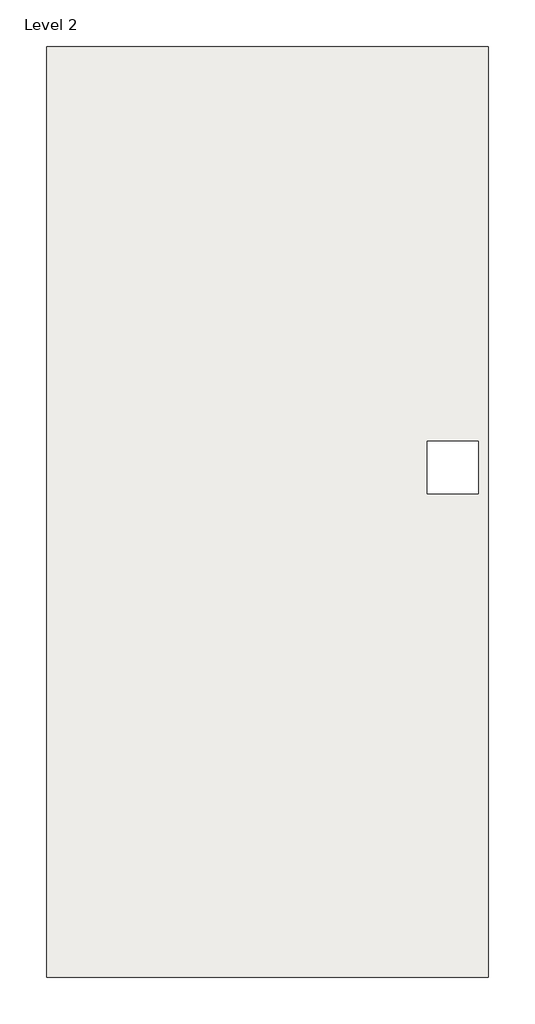
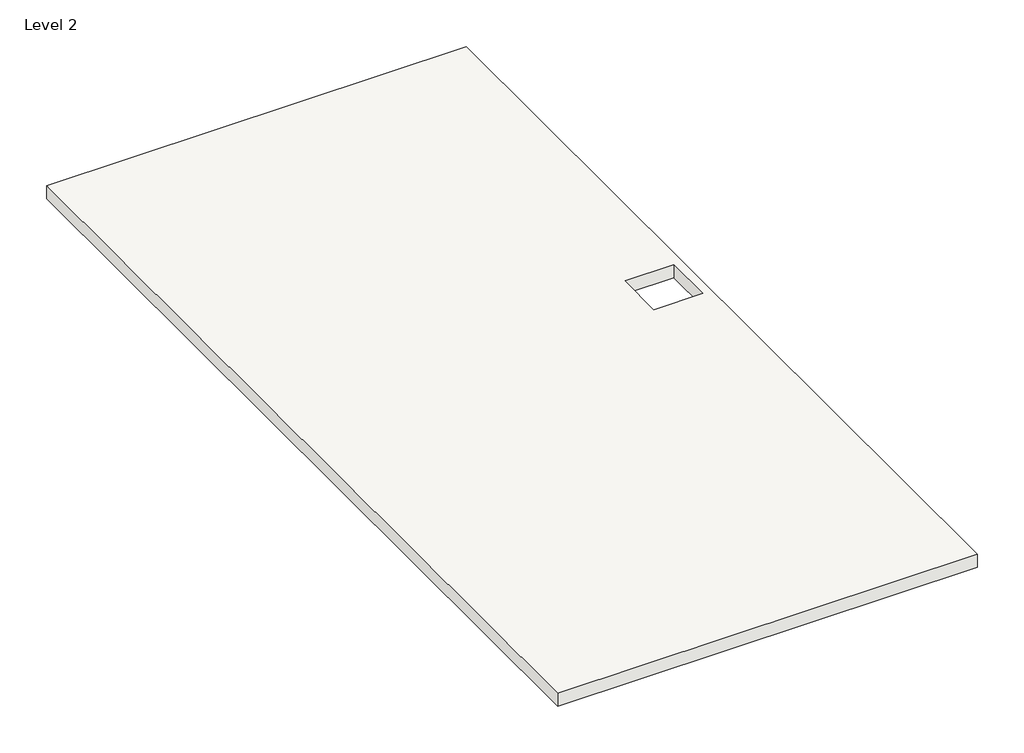
# One storey: 1 roof.
"""IFC4 building model written with IfcOpenShell, lengths in millimetres."""

from ifc_helpers import new_model, si_unit, frame, origin, place, context, project, spatial, polyline, outline, extrude, element, save

model = new_model("IFC4")

# Units and contexts
model_context = context("Model", 3, world=origin())
ifc_project = project(units=[si_unit("LENGTHUNIT", "METRE", prefix="MILLI")], contexts=[model_context])

# Site, building, storey
site = spatial("IfcSite", under=ifc_project)
building = spatial("IfcBuilding", under=site)
storey = spatial("IfcBuildingStorey", under=building, Name="Level 2", Elevation=3048.0)

# Roof
placement = place(None, origin())
element("IfcRoof", 1, ObjectType="Generic - 12\"", at=placement, inside=storey, context=model_context, shape_type="SweptSolid", body=[
    extrude(outline(polyline([(-11802.0976606, 13853.2271763), (-2454.8976606, 13853.2271763), (-2454.8976606, -5857.1728237), (-11802.0976606, -5857.1728237), (-11802.0976606, 13853.2271763)]), holes=[polyline([(-2658.0976606, 4389.4901868), (-2658.0976606, 5496.6271763), (-3743.9476606, 5496.6271763), (-3743.9476606, 4389.4901868), (-2658.0976606, 4389.4901868)])]), frame((0.0, 0.0, 3048.0), z_axis=(0.0, 0.0, 1.0), x_axis=(1.0, 0.0, 0.0)), (0.0, 0.0, 1.0), 304.8),
])

save(model, "model.ifc")

# Revit data of these elements
# Type "Generic - 12\""
#   Assembly Code = "B1020"
#   Layers, outside or top first: 1' - 0" "Brick, Soldier Course" (function 1)
# Element 1 (IfcRoof, "Generic - 12\"")
#   built-in parameter 1001705 = 11 (stored number, unit not read)
#   built-in parameter 1001710 = 33615
#   Phase Created = New Construction
#   Materials on its faces: "Brick, Soldier Course"
# Materials
#   "Brick, Soldier Course": class "Masonry", colour RGB 170 98 104, transparency 0, Description = "Common brick soldier coursed", Cost = 0
